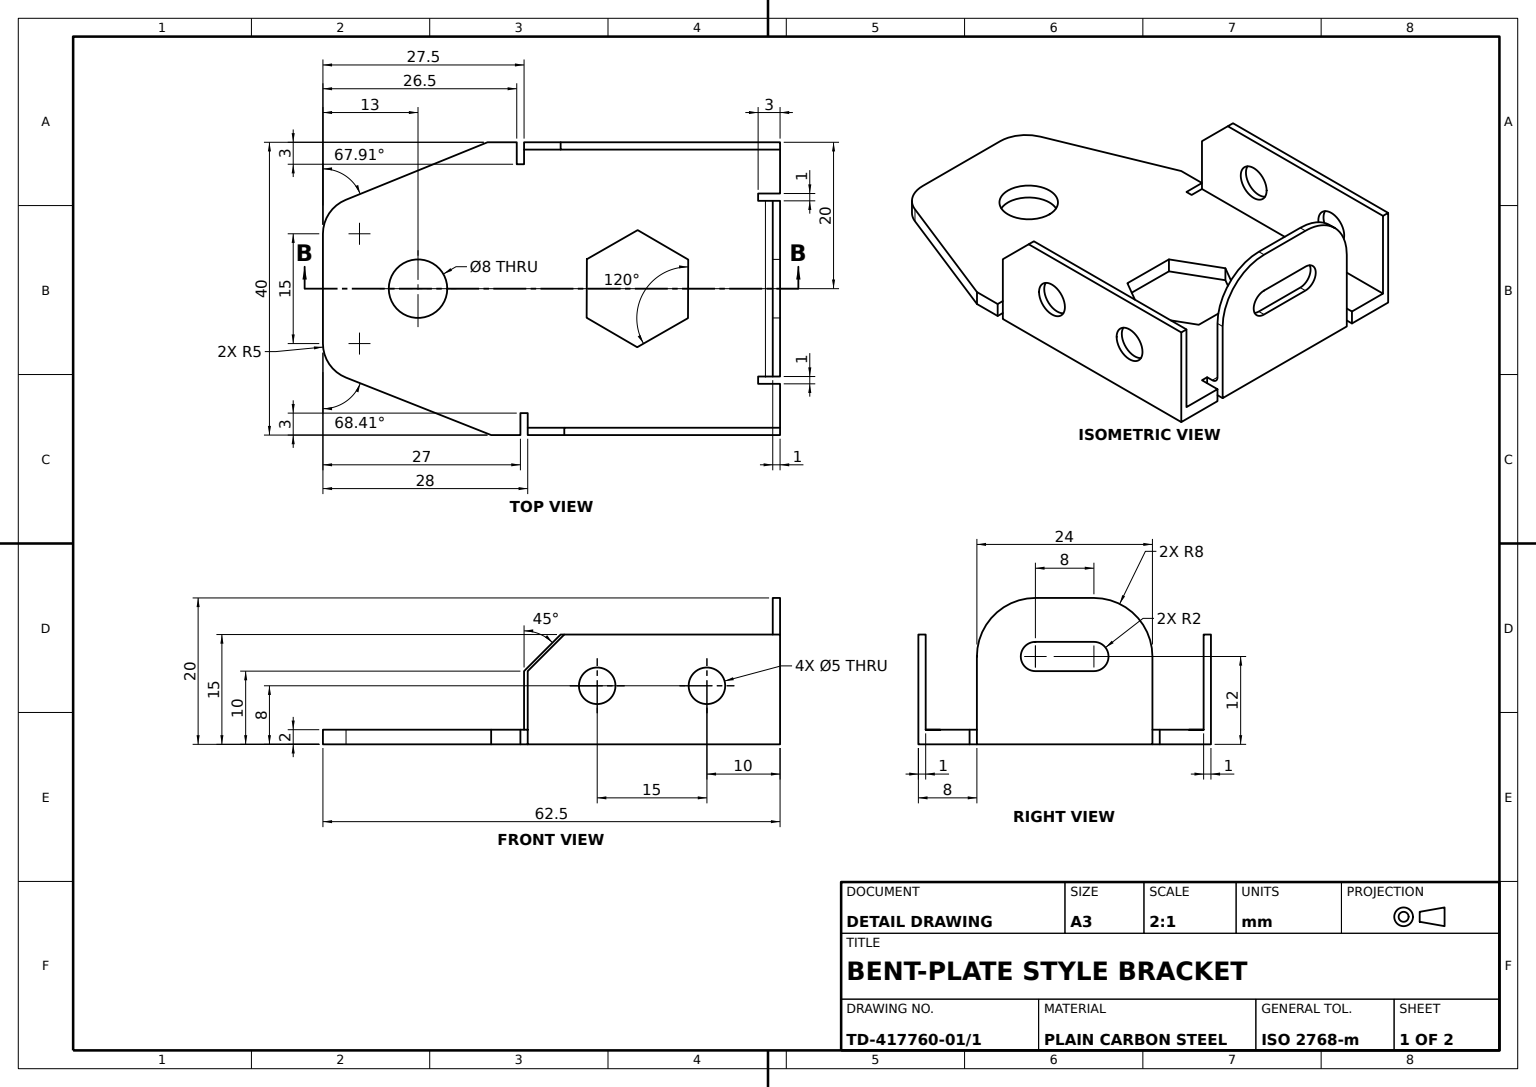
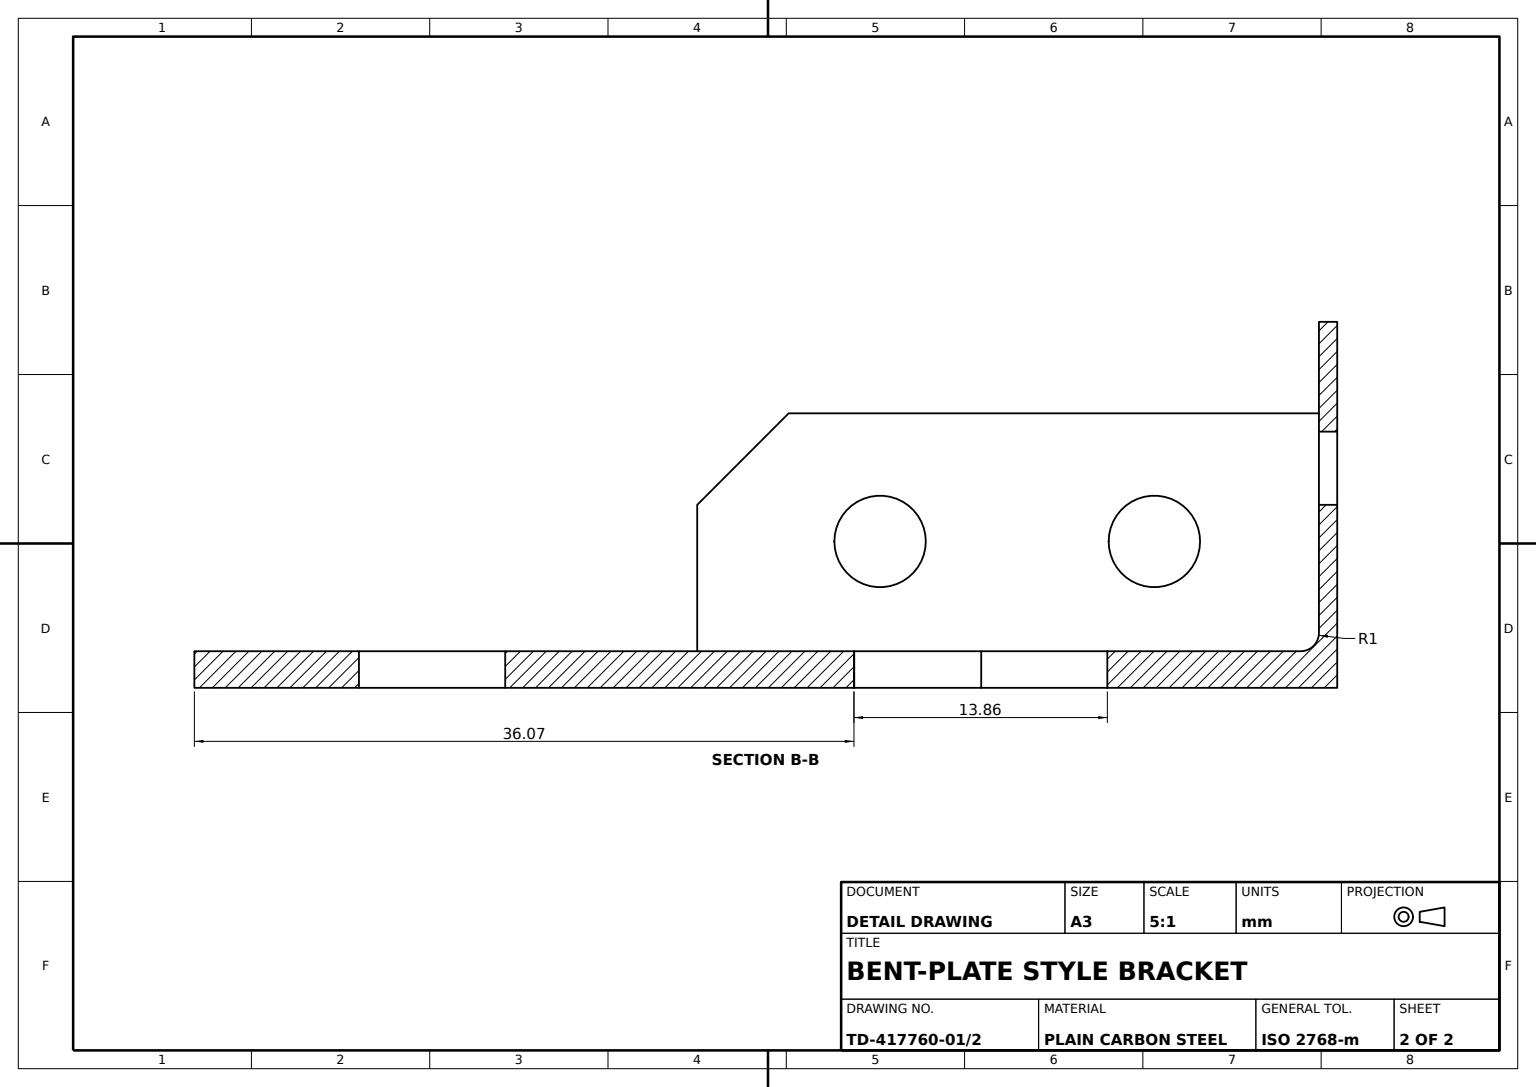
SolidWorks part; units mm, degrees
material "Plain Carbon Steel"
ref_plane "Front Plane" through (0, 0, 0) normal (0, 0, 1) x (1, 0, 0)
ref_plane "Top Plane" through (0, 0, 0) normal (0, 1, 0) x (1, 0, 0)
ref_plane "Right Plane" through (0, 0, 0) normal (1, 0, 0) x (0, 0, -1)
sketch "Base Plate Profile" plane through (0, 0, 0) normal (0, 1, 0) x (1, 0, 0)
  line L0 (-20, 0) -> (-13, 0)
  line L1 (12, -0.5) -> (12, -3)
  line L2 (-12, -0.5) -> (12, -0.5)
  line L3 (-12, 0.5) -> (12, 0.5)
  line L4 (-12, 0.5) -> (-12, -0.5)
  line L5 (12, 0.5) -> (12, -0.5)
  line L6 (13, 0) -> (20, 0)
  line L7 (-20, 0.5) -> (20, 0.5) construction
  line L8 (-20, -0.5) -> (20, -0.5) construction
  line L9 (12, -3) -> (13, -3)
  line L10 (-20, 0) -> (20, 0) construction
  line L11 (13, -3) -> (13, 0)
  line L12 (-12, -0.5) -> (-12, -3)
  line L13 (-12, -3) -> (-13, -3)
  line L14 (-13, -3) -> (-13, 0)
  line L15 (-20, 0) -> (-20, -35)
  line L16 (-20, -35) -> (-17, -35)
  line L17 (-17, -35) -> (-17, -36)
  line L18 (-17, -36) -> (-20, -36)
  line L19 (-20, -36) -> (-20, -40)
  line L20 (20, 0) -> (20, -34.5)
  line L21 (20, -34.5) -> (17, -34.5)
  line L22 (17, -34.5) -> (17, -35.5)
  line L23 (17, -35.5) -> (20, -35.5)
  line L24 (20, -35.5) -> (20, -39.5)
  line L25 (19, 0) -> (19, -34.5)
  line L26 (-19, 0) -> (-19, -35)
  line L27 (-7.5, -62.5) -> (7.5, -62.5)
  line L29 (12.1492, -59.3397) -> (20, -39.5)
  line L30 (3.9732, -26.4437) -> (8, -19.5309)
  line L31 (-12.1329, -59.3806) -> (-20, -40)
  line L32 (8, -19.5309) -> (4.0268, -12.5872)
  line L33 (4.0268, -12.5872) -> (-3.9732, -12.5563)
  line L34 (-3.9732, -12.5563) -> (-8, -19.4691)
  line L35 (-8, -19.4691) -> (-4.0268, -26.4128)
  line L36 (-4.0268, -26.4128) -> (3.9732, -26.4437)
  arc A0 (7.5, -62.5) -> (12.1492, -59.3397) centre (7.5, -57.5) ccw
  arc A1 (-12.1329, -59.3806) -> (-7.5, -62.5) centre (-7.5, -57.5) ccw
  circle A2 centre (0, -49.5) radius 4
  circle A3 centre (0, -19.5) radius 6.9283 construction
  point P4 (0, 0)
  point P8 (0, 0)
  point P37 (0, -62.5)
  dimension "D21" = 5
  dimension "D22" = 5
  dimension "D23" = 8
  dimension "D1" = 20
  dimension "D2" = 0.5
  dimension "D4" = 1
  dimension "D6" = 63
  dimension "D7" = 7.5
  dimension "D8" = 35
  dimension "D9" = 24
  dimension "D10" = 3
  dimension "D11" = 3
  dimension "D12" = 1
  dimension "D13" = 1
  dimension "D14" = 40
  dimension "D15" = 4
  dimension "D16" = 3
  dimension "D17" = 1
  dimension "D18" = 1
  dimension "D19" = 3
  dimension "D20" = 4
  dimension "D24" = 13
  dimension "D25" = 3
  dimension "D26" = 16
  dimension "D27" = 20
  dimension "D28" = 20
  dimension "D29" = 12
  dimension "D30" = 3
  dimension "D31" = 0.221
  dimension "D3" = 0.5
  dimension "D5" = 1
extrude "Base Plate 2mm" add sketch "Base Plate Profile" along normal blind 2 contours L31 A1 L27 A0 L29 L24 L23 L22 L21 L25 L6 L11 L9 L1 L2 L12 L13 L14 L0 L26 L16 L17 L18 L19 A2 L36 L35 L34 L33 L32 L30 | L26 L0 L15 L16 | L5 L3 L4 L2 | L6 L25 L21 L20
sketch "Tab Seat Recess Sketch" plane through (0, 0, -0.5) normal (0, 0, -1) x (-1, 0, 0)
  line L0 (-12, 2) -> (-12, 0)
  line L1 (-12, 0) -> (12, 0)
  line L2 (12, 0) -> (12, 2)
  line L3 (12, 2) -> (-12, 2)
extrude "Tab Seat Recess 0.5mm" cut sketch "Tab Seat Recess Sketch" against normal blind 0.5
sketch "Side Flanges Sketch" plane through (20, 0, 0) normal (1, 0, 0) x (0, 0, -1)
  line L0 (-34.5, 2) -> (-34.5, 0)
  line L1 (-34.5, 0) -> (0, 0)
  line L2 (0, 0) -> (0, 2)
  line L3 (0, 2) -> (-34.5, 2)
  line L4 (-34.5, 2) -> (-34.5, 10)
  line L5 (0, 2) -> (0, 15)
  line L6 (0, 15) -> (-29.5, 15)
  line L7 (-29.5, 15) -> (-34.5, 10)
  line M4 (-34.5, 0) -> (0, 0)
  line M5 (0, 0) -> (0, 2)
  line M6 (0, 2) -> (-34.5, 2)
  line M7 (-34.5, 2) -> (-34.5, 0)
  dimension "D1" = 8
  dimension "D2" = 29.5
  dimension "D3" = 13
extrude "Side Flanges" add sketch "Side Flanges Sketch" against normal blind 1 contours L6 L7 L4 L5 M6 | M7 M4 M5 M6
sketch "Flange Extension Sketch" plane through (-20, 0, 0) normal (-1, 0, 0) x (0, 0, 1)
  line L0 (0, 15) -> (0, 0)
  line L1 (0, 0) -> (35, 0)
  line L2 (35, 0) -> (35, 10)
  line L3 (35, 10) -> (30, 15)
  line L4 (30, 15) -> (0, 15)
  line L5 (0, 0) -> (35, 0) construction
  dimension "D1" = 5
  dimension "D2" = 10
extrude "Flange Extension" add sketch "Flange Extension Sketch" against normal blind 1
sketch "Rear Tab Sketch" plane through (0, 0, 0) normal (0, 0, -1) x (-1, 0, 0)
  line L1 (-12, 0) -> (12, 0)
  line L2 (-12, 0) -> (-12, 20)
  line L3 (-12, 20) -> (12, 20)
  line L4 (12, 0) -> (12, 20)
  dimension "D1" = 24
  dimension "D2" = 20
extrude "Rear Tab 24x20" add sketch "Rear Tab Sketch" against normal blind 1
fillet "Rear Tab Corner Round R8" radius 8 2 edges at (-12, 20, 0.5) (12, 20, 0.5)
sketch "Tab Slot Sketch" plane through (0, 0, 1) normal (0, 0, 1) x (1, 0, 0)
  line L1 (-3.9989, 12) -> (3.9989, 12) construction
  line L2 (-3.9989, 14) -> (3.9989, 14)
  line L3 (-3.9989, 10) -> (3.9989, 10)
  line L4 (-4, 20) -> (4, 20) construction
  arc A0 (-3.9989, 14) -> (-3.9989, 10) centre (-3.9989, 12) ccw
  arc A1 (3.9989, 10) -> (3.9989, 14) centre (3.9989, 12) ccw
  point P0 (0, 12)
  point P3 (0, 12)
  dimension "D3" = 2
  dimension "D4" = 3.9989
  dimension "D1" = 3.9989
  dimension "D2" = 8
extrude "Tab Slot" cut sketch "Tab Slot Sketch" against normal blind 2
fillet "Tab Root Fillet R1" radius 1 1 edges at (0, 2, 1)
sketch "Flange Cross Holes Sketch" plane through (-20, 0, 0) normal (-1, 0, 0) x (0, 0, 1)
  line L0 (0, 15) -> (0, 0) construction
  line L2 (0, 0) -> (35, 0) construction
  circle A0 centre (10, 8) radius 2.5
  circle A1 centre (25, 8) radius 2.5
  dimension "D1" = 5
  dimension "D2" = 5
  dimension "D3" = 10
  dimension "D4" = 15
  dimension "D5" = 8
  dimension "D6" = 8
extrude "Flange Cross Holes" cut sketch "Flange Cross Holes Sketch" against normal blind 50
